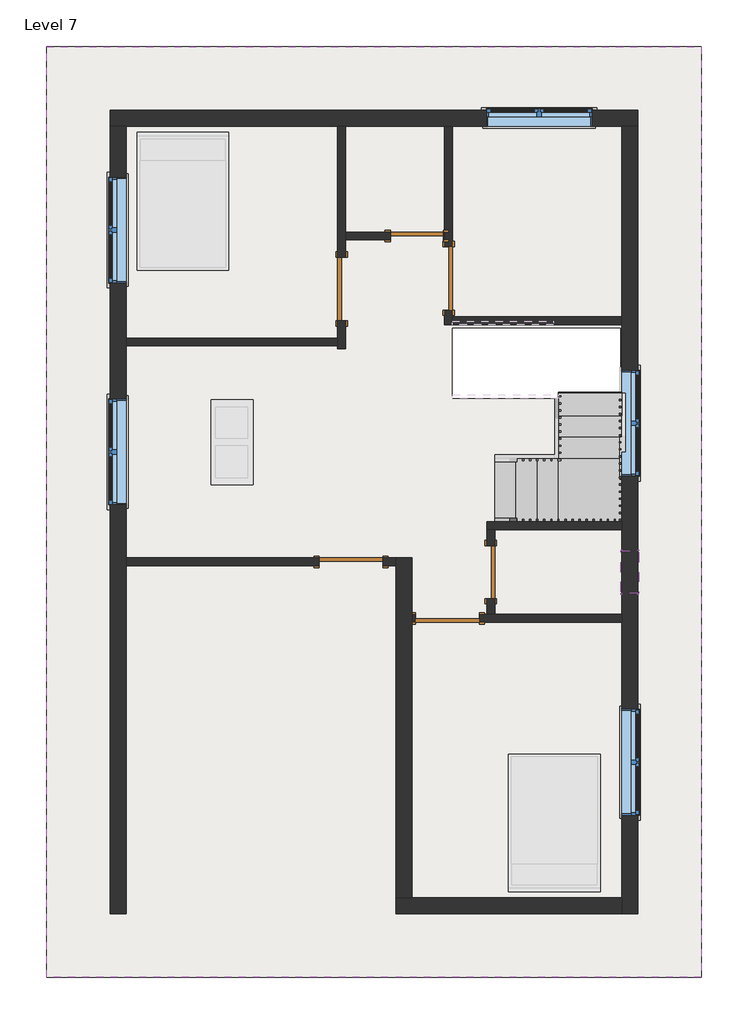
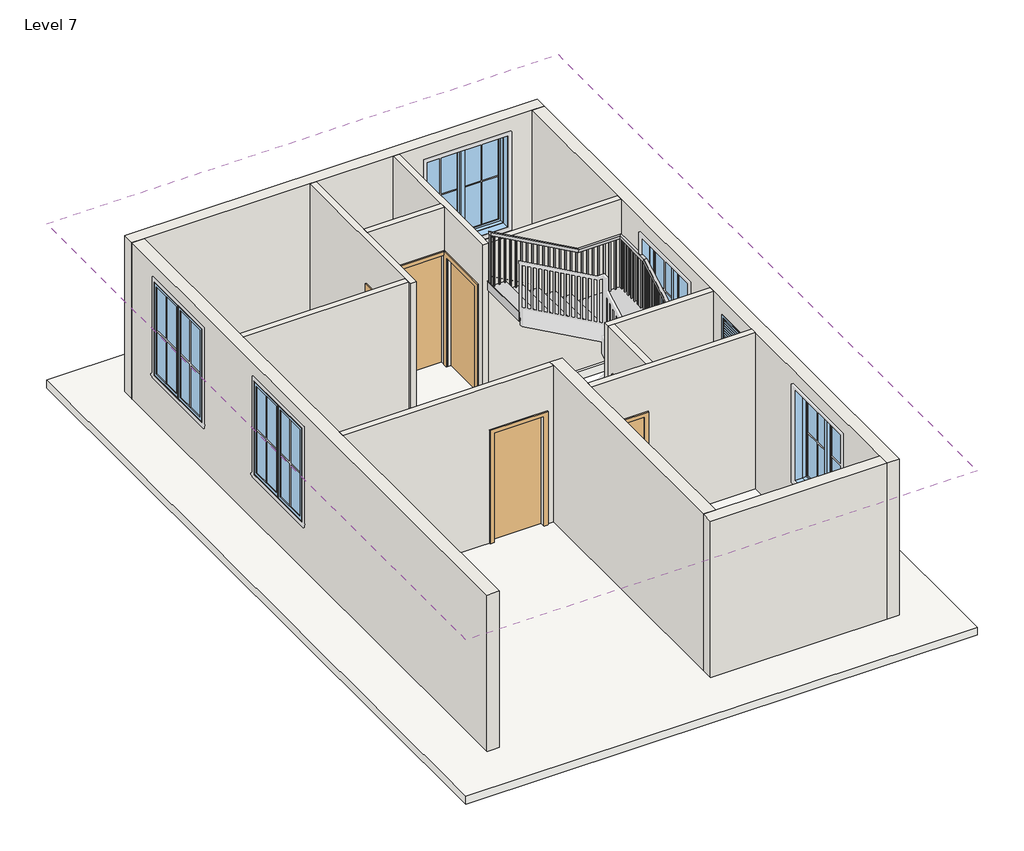
# One storey, part 1 of 2: 14 walls, 6 doors, 6 windows, 2 roofs, 1 railing, 1 slab, 1 stair flight.
"""IFC4 building model written with IfcOpenShell, lengths in millimetres."""

from ifc_helpers import new_model, si_unit, frame, origin, place, context, project, spatial, polyline, outline, extrude, faceted_brep, transform, mapped, element, save
from components import door_214872d5, door_78caadf7, single_flush_door_3_e5f9f3c4, single_flush_door_3_305aa2a5, stair_flight_68b2e5de, window_casement_double_win_5_f93960c7, window_f2d8fef0

model = new_model("IFC4")

# Units and contexts
model_context = context("Model", 3, world=origin())
ifc_project = project(units=[si_unit("LENGTHUNIT", "METRE", prefix="MILLI")], contexts=[model_context])

# Site, building, storey
site = spatial("IfcSite", under=ifc_project)
building = spatial("IfcBuilding", under=site)
storey = spatial("IfcBuildingStorey", under=building, Name="Level 7", Elevation=16002.0)

# Doors
placement = place(None, origin())
door_shape = door_214872d5(model_context)
element("IfcDoor", 1, ObjectType="Single-Flush : DOOR 2'6\"", at=placement, inside=storey, context=model_context, shape_type="MappedRepresentation", body=[
    mapped(door_shape, transform((-185.4325206, 3926.3629493, 16002.0), x_axis=(1.0, 0.0, 0.0), y_axis=(0.0, 1.0, 0.0), z_axis=(0.0, 0.0, 1.0))),
])
door_2_shape = door_78caadf7(model_context)
element("IfcDoor", 2, ObjectType="Single-Flush : DOOR 2'6\"", at=placement, inside=storey, context=model_context, shape_type="MappedRepresentation", body=[
    mapped(door_2_shape, transform((881.3674794, -905.9870507, 16002.0), x_axis=(0.0, 1.0, 0.0), y_axis=(-1.0, 0.0, 0.0), z_axis=(0.0, 0.0, 1.0))),
])
single_flush_door_3_shape = single_flush_door_3_e5f9f3c4(model_context)
element("IfcDoor", 3, ObjectType="Single-Flush : DOOR 3'", at=placement, inside=storey, context=model_context, shape_type="MappedRepresentation", body=[
    mapped(single_flush_door_3_shape, transform((271.7674794, 3316.7629493, 16002.0), x_axis=(0.0, -1.0, 0.0), y_axis=(1.0, 0.0, 0.0), z_axis=(0.0, 0.0, 1.0))),
])
element("IfcDoor", 4, ObjectType="Single-Flush : DOOR 3'", at=placement, inside=storey, context=model_context, shape_type="MappedRepresentation", body=[
    mapped(single_flush_door_3_shape, transform((255.8924794, -1572.7370507, 16002.0), x_axis=(-1.0, 0.0, 0.0), y_axis=(0.0, -1.0, 0.0), z_axis=(0.0, 0.0, 1.0))),
])
single_flush_door_3_2_shape = single_flush_door_3_305aa2a5(model_context)
element("IfcDoor", 5, ObjectType="Single-Flush : DOOR 3'", at=placement, inside=storey, context=model_context, shape_type="MappedRepresentation", body=[
    mapped(single_flush_door_3_2_shape, transform((-1264.9325206, 3164.3629493, 16002.0), x_axis=(0.0, -1.0, 0.0), y_axis=(1.0, 0.0, 0.0), z_axis=(0.0, 0.0, 1.0))),
])
element("IfcDoor", 6, ObjectType="Single-Flush : DOOR 3'6\"", at=placement, inside=storey, context=model_context, shape_type="MappedRepresentation", body=[
    mapped(single_flush_door_3_shape, transform((-1131.5825206, -759.9370507, 16002.0), x_axis=(1.0, 0.0, 0.0), y_axis=(0.0, 1.0, 0.0), z_axis=(0.0, 0.0, 1.0))),
])

# Railing
element("IfcRailing", 7, ObjectType="Handrail - Rectangular", at=placement, inside=storey, context=model_context, shape_type="SolidModel", body=[
    faceted_brep([(938.5174794, -131.2870507, 17085.7333333), (938.5174794, -131.2870507, 17027.620221), (938.5174794, -182.0870507, 17027.620221), (938.5174794, -182.0870507, 17085.7333333), (2005.3174794, -131.2870507, 17678.4), (2018.4810817, -131.2870507, 17627.6), (2018.4810817, -182.0870507, 17627.6), (2005.3174794, -182.0870507, 17678.4), (2716.5174794, -131.2870507, 17678.4), (2716.5174794, -131.2870507, 17627.6), (2767.3174794, -182.0870507, 17627.6), (2767.3174794, -182.0870507, 17678.4), (2716.5174794, 579.9129493, 17678.4), (2716.5174794, 593.0765516, 17627.6), (2767.3174794, 593.0765516, 17627.6), (2767.3174794, 579.9129493, 17678.4), (2716.5174794, 1843.5629493, 18380.4277778), (2716.5174794, 1856.7265516, 18329.6277778), (2767.3174794, 1856.7265516, 18329.6277778), (2767.3174794, 1843.5629493, 18380.4277778), (2716.5174794, 2599.2129493, 18380.4277778), (2716.5174794, 2599.2129493, 18329.6277778), (2767.3174794, 2650.0129493, 18329.6277778), (2767.3174794, 2650.0129493, 18380.4277778), (1960.8674794, 2599.2129493, 18380.4277778), (1947.7038772, 2599.2129493, 18329.6277778), (1947.7038772, 2650.0129493, 18329.6277778), (1960.8674794, 2650.0129493, 18380.4277778), (328.9174794, 2599.2129493, 19287.0666667), (328.9174794, 2650.0129493, 19287.0666667), (328.9174794, 2650.0129493, 19228.9535543), (328.9174794, 2599.2129493, 19228.9535543)], [[[0, 1, 2, 3]], [[1, 0, 4, 5]], [[2, 1, 5, 6]], [[3, 2, 6, 7]], [[0, 3, 7, 4]], [[5, 4, 8, 9]], [[6, 5, 9, 10]], [[7, 6, 10, 11]], [[4, 7, 11, 8]], [[9, 8, 12, 13]], [[10, 9, 13, 14]], [[11, 10, 14, 15]], [[8, 11, 15, 12]], [[13, 12, 16, 17]], [[14, 13, 17, 18]], [[15, 14, 18, 19]], [[12, 15, 19, 16]], [[17, 16, 20, 21]], [[18, 17, 21, 22]], [[19, 18, 22, 23]], [[16, 19, 23, 20]], [[21, 20, 24, 25]], [[22, 21, 25, 26]], [[23, 22, 26, 27]], [[20, 23, 27, 24]], [[28, 29, 30, 31]], [[25, 24, 28, 31]], [[26, 25, 31, 30]], [[27, 26, 30, 29]], [[24, 27, 29, 28]]]),
    extrude(outline(polyline([(19181.3285543, 414.6424794), (19191.9118876, 395.5924794), (18203.3333333, 395.5924794), (18203.3333333, 414.6424794), (19181.3285543, 414.6424794)])), frame((0.0, 2615.0879493, 0.0), z_axis=(0.0, 1.0, 0.0), x_axis=(0.0, 0.0, 1.0)), (0.0, 0.0, 1.0), 19.05),
    extrude(outline(polyline([(19124.8841099, 516.2424794), (19135.4674432, 497.1924794), (18203.3333333, 497.1924794), (18203.3333333, 516.2424794), (19124.8841099, 516.2424794)])), frame((0.0, 2615.0879493, 0.0), z_axis=(0.0, 1.0, 0.0), x_axis=(0.0, 0.0, 1.0)), (0.0, 0.0, 1.0), 19.05),
    extrude(outline(polyline([(19068.4396654, 617.8424794), (19079.0229988, 598.7924794), (18203.3333333, 598.7924794), (18203.3333333, 617.8424794), (19068.4396654, 617.8424794)])), frame((0.0, 2615.0879493, 0.0), z_axis=(0.0, 1.0, 0.0), x_axis=(0.0, 0.0, 1.0)), (0.0, 0.0, 1.0), 19.05),
    extrude(outline(polyline([(19011.995221, 719.4424794), (19022.5785543, 700.3924794), (18034.0, 700.3924794), (18034.0, 719.4424794), (19011.995221, 719.4424794)])), frame((0.0, 2615.0879493, 0.0), z_axis=(0.0, 1.0, 0.0), x_axis=(0.0, 0.0, 1.0)), (0.0, 0.0, 1.0), 19.05),
    extrude(outline(polyline([(18955.5507765, 821.0424794), (18966.1341099, 801.9924794), (18034.0, 801.9924794), (18034.0, 821.0424794), (18955.5507765, 821.0424794)])), frame((0.0, 2615.0879493, 0.0), z_axis=(0.0, 1.0, 0.0), x_axis=(0.0, 0.0, 1.0)), (0.0, 0.0, 1.0), 19.05),
    extrude(outline(polyline([(18899.1063321, 922.6424794), (18909.6896654, 903.5924794), (18034.0, 903.5924794), (18034.0, 922.6424794), (18899.1063321, 922.6424794)])), frame((0.0, 2615.0879493, 0.0), z_axis=(0.0, 1.0, 0.0), x_axis=(0.0, 0.0, 1.0)), (0.0, 0.0, 1.0), 19.05),
    extrude(outline(polyline([(18842.6618876, 1024.2424794), (18853.245221, 1005.1924794), (17864.6666667, 1005.1924794), (17864.6666667, 1024.2424794), (18842.6618876, 1024.2424794)])), frame((0.0, 2615.0879493, 0.0), z_axis=(0.0, 1.0, 0.0), x_axis=(0.0, 0.0, 1.0)), (0.0, 0.0, 1.0), 19.05),
    extrude(outline(polyline([(18786.2174432, 1125.8424794), (18796.8007765, 1106.7924794), (17864.6666667, 1106.7924794), (17864.6666667, 1125.8424794), (18786.2174432, 1125.8424794)])), frame((0.0, 2615.0879493, 0.0), z_axis=(0.0, 1.0, 0.0), x_axis=(0.0, 0.0, 1.0)), (0.0, 0.0, 1.0), 19.05),
    extrude(outline(polyline([(18729.7729988, 1227.4424794), (18740.3563321, 1208.3924794), (17864.6666667, 1208.3924794), (17864.6666667, 1227.4424794), (18729.7729988, 1227.4424794)])), frame((0.0, 2615.0879493, 0.0), z_axis=(0.0, 1.0, 0.0), x_axis=(0.0, 0.0, 1.0)), (0.0, 0.0, 1.0), 19.05),
    extrude(outline(polyline([(18673.3285543, 1329.0424794), (18683.9118876, 1309.9924794), (17695.3333333, 1309.9924794), (17695.3333333, 1329.0424794), (18673.3285543, 1329.0424794)])), frame((0.0, 2615.0879493, 0.0), z_axis=(0.0, 1.0, 0.0), x_axis=(0.0, 0.0, 1.0)), (0.0, 0.0, 1.0), 19.05),
    extrude(outline(polyline([(18616.8841099, 1430.6424794), (18627.4674432, 1411.5924794), (17695.3333333, 1411.5924794), (17695.3333333, 1430.6424794), (18616.8841099, 1430.6424794)])), frame((0.0, 2615.0879493, 0.0), z_axis=(0.0, 1.0, 0.0), x_axis=(0.0, 0.0, 1.0)), (0.0, 0.0, 1.0), 19.05),
    extrude(outline(polyline([(18560.4396654, 1532.2424794), (18571.0229988, 1513.1924794), (17695.3333333, 1513.1924794), (17695.3333333, 1532.2424794), (18560.4396654, 1532.2424794)])), frame((0.0, 2615.0879493, 0.0), z_axis=(0.0, 1.0, 0.0), x_axis=(0.0, 0.0, 1.0)), (0.0, 0.0, 1.0), 19.05),
    extrude(outline(polyline([(18503.995221, 1633.8424794), (18514.5785543, 1614.7924794), (17526.0, 1614.7924794), (17526.0, 1633.8424794), (18503.995221, 1633.8424794)])), frame((0.0, 2615.0879493, 0.0), z_axis=(0.0, 1.0, 0.0), x_axis=(0.0, 0.0, 1.0)), (0.0, 0.0, 1.0), 19.05),
    extrude(outline(polyline([(18447.5507765, 1735.4424794), (18458.1341099, 1716.3924794), (17526.0, 1716.3924794), (17526.0, 1735.4424794), (18447.5507765, 1735.4424794)])), frame((0.0, 2615.0879493, 0.0), z_axis=(0.0, 1.0, 0.0), x_axis=(0.0, 0.0, 1.0)), (0.0, 0.0, 1.0), 19.05),
    extrude(outline(polyline([(18391.1063321, 1837.0424794), (18401.6896654, 1817.9924794), (17526.0, 1817.9924794), (17526.0, 1837.0424794), (18391.1063321, 1837.0424794)])), frame((0.0, 2615.0879493, 0.0), z_axis=(0.0, 1.0, 0.0), x_axis=(0.0, 0.0, 1.0)), (0.0, 0.0, 1.0), 19.05),
    extrude(outline(polyline([(18334.6618876, 1938.6424794), (18345.245221, 1919.5924794), (17356.6666667, 1919.5924794), (17356.6666667, 1938.6424794), (18334.6618876, 1938.6424794)])), frame((0.0, 2615.0879493, 0.0), z_axis=(0.0, 1.0, 0.0), x_axis=(0.0, 0.0, 1.0)), (0.0, 0.0, 1.0), 19.05),
    extrude(outline(polyline([(2040.2424794, 2634.1379493), (2040.2424794, 2615.0879493), (2021.1924794, 2615.0879493), (2021.1924794, 2634.1379493), (2040.2424794, 2634.1379493)])), frame((0.0, 0.0, 17356.6666667), z_axis=(0.0, 0.0, 1.0), x_axis=(1.0, 0.0, 0.0)), (0.0, 0.0, 1.0), 972.9611111),
    extrude(outline(polyline([(2141.8424794, 2634.1379493), (2141.8424794, 2615.0879493), (2122.7924794, 2615.0879493), (2122.7924794, 2634.1379493), (2141.8424794, 2634.1379493)])), frame((0.0, 0.0, 17356.6666667), z_axis=(0.0, 0.0, 1.0), x_axis=(1.0, 0.0, 0.0)), (0.0, 0.0, 1.0), 972.9611111),
    extrude(outline(polyline([(2243.4424794, 2634.1379493), (2243.4424794, 2615.0879493), (2224.3924794, 2615.0879493), (2224.3924794, 2634.1379493), (2243.4424794, 2634.1379493)])), frame((0.0, 0.0, 17356.6666667), z_axis=(0.0, 0.0, 1.0), x_axis=(1.0, 0.0, 0.0)), (0.0, 0.0, 1.0), 972.9611111),
    extrude(outline(polyline([(2345.0424794, 2634.1379493), (2345.0424794, 2615.0879493), (2325.9924794, 2615.0879493), (2325.9924794, 2634.1379493), (2345.0424794, 2634.1379493)])), frame((0.0, 0.0, 17356.6666667), z_axis=(0.0, 0.0, 1.0), x_axis=(1.0, 0.0, 0.0)), (0.0, 0.0, 1.0), 972.9611111),
    extrude(outline(polyline([(2446.6424794, 2634.1379493), (2446.6424794, 2615.0879493), (2427.5924794, 2615.0879493), (2427.5924794, 2634.1379493), (2446.6424794, 2634.1379493)])), frame((0.0, 0.0, 17356.6666667), z_axis=(0.0, 0.0, 1.0), x_axis=(1.0, 0.0, 0.0)), (0.0, 0.0, 1.0), 972.9611111),
    extrude(outline(polyline([(2548.2424794, 2634.1379493), (2548.2424794, 2615.0879493), (2529.1924794, 2615.0879493), (2529.1924794, 2634.1379493), (2548.2424794, 2634.1379493)])), frame((0.0, 0.0, 17356.6666667), z_axis=(0.0, 0.0, 1.0), x_axis=(1.0, 0.0, 0.0)), (0.0, 0.0, 1.0), 972.9611111),
    extrude(outline(polyline([(2649.8424794, 2634.1379493), (2649.8424794, 2615.0879493), (2630.7924794, 2615.0879493), (2630.7924794, 2634.1379493), (2649.8424794, 2634.1379493)])), frame((0.0, 0.0, 17356.6666667), z_axis=(0.0, 0.0, 1.0), x_axis=(1.0, 0.0, 0.0)), (0.0, 0.0, 1.0), 972.9611111),
    extrude(outline(polyline([(2751.4424794, 2576.9879493), (2732.3924794, 2576.9879493), (2732.3924794, 2596.0379493), (2751.4424794, 2596.0379493), (2751.4424794, 2576.9879493)])), frame((0.0, 0.0, 17356.6666667), z_axis=(0.0, 0.0, 1.0), x_axis=(1.0, 0.0, 0.0)), (0.0, 0.0, 1.0), 972.9611111),
    extrude(outline(polyline([(2751.4424794, 2475.3879493), (2732.3924794, 2475.3879493), (2732.3924794, 2494.4379493), (2751.4424794, 2494.4379493), (2751.4424794, 2475.3879493)])), frame((0.0, 0.0, 17356.6666667), z_axis=(0.0, 0.0, 1.0), x_axis=(1.0, 0.0, 0.0)), (0.0, 0.0, 1.0), 972.9611111),
    extrude(outline(polyline([(2751.4424794, 2373.7879493), (2732.3924794, 2373.7879493), (2732.3924794, 2392.8379493), (2751.4424794, 2392.8379493), (2751.4424794, 2373.7879493)])), frame((0.0, 0.0, 17356.6666667), z_axis=(0.0, 0.0, 1.0), x_axis=(1.0, 0.0, 0.0)), (0.0, 0.0, 1.0), 972.9611111),
    extrude(outline(polyline([(2751.4424794, 2272.1879493), (2732.3924794, 2272.1879493), (2732.3924794, 2291.2379493), (2751.4424794, 2291.2379493), (2751.4424794, 2272.1879493)])), frame((0.0, 0.0, 17356.6666667), z_axis=(0.0, 0.0, 1.0), x_axis=(1.0, 0.0, 0.0)), (0.0, 0.0, 1.0), 972.9611111),
    extrude(outline(polyline([(2751.4424794, 2170.5879493), (2732.3924794, 2170.5879493), (2732.3924794, 2189.6379493), (2751.4424794, 2189.6379493), (2751.4424794, 2170.5879493)])), frame((0.0, 0.0, 17356.6666667), z_axis=(0.0, 0.0, 1.0), x_axis=(1.0, 0.0, 0.0)), (0.0, 0.0, 1.0), 972.9611111),
    extrude(outline(polyline([(2751.4424794, 2068.9879493), (2732.3924794, 2068.9879493), (2732.3924794, 2088.0379493), (2751.4424794, 2088.0379493), (2751.4424794, 2068.9879493)])), frame((0.0, 0.0, 17356.6666667), z_axis=(0.0, 0.0, 1.0), x_axis=(1.0, 0.0, 0.0)), (0.0, 0.0, 1.0), 972.9611111),
    extrude(outline(polyline([(2751.4424794, 1967.3879493), (2732.3924794, 1967.3879493), (2732.3924794, 1986.4379493), (2751.4424794, 1986.4379493), (2751.4424794, 1967.3879493)])), frame((0.0, 0.0, 17356.6666667), z_axis=(0.0, 0.0, 1.0), x_axis=(1.0, 0.0, 0.0)), (0.0, 0.0, 1.0), 972.9611111),
    extrude(outline(polyline([(2751.4424794, 1865.7879493), (2732.3924794, 1865.7879493), (2732.3924794, 1884.8379493), (2751.4424794, 1884.8379493), (2751.4424794, 1865.7879493)])), frame((0.0, 0.0, 17356.6666667), z_axis=(0.0, 0.0, 1.0), x_axis=(1.0, 0.0, 0.0)), (0.0, 0.0, 1.0), 972.9611111),
    extrude(outline(polyline([(1764.1879493, 18278.2174432), (1783.2379493, 18288.8007765), (1783.2379493, 17356.6666667), (1764.1879493, 17356.6666667), (1764.1879493, 18278.2174432)])), frame((2732.3924794, 0.0, 0.0), z_axis=(1.0, 0.0, 0.0), x_axis=(0.0, 1.0, 0.0)), (0.0, 0.0, 1.0), 19.05),
    extrude(outline(polyline([(1662.5879493, 18221.7729988), (1681.6379493, 18232.3563321), (1681.6379493, 17356.6666667), (1662.5879493, 17356.6666667), (1662.5879493, 18221.7729988)])), frame((2732.3924794, 0.0, 0.0), z_axis=(1.0, 0.0, 0.0), x_axis=(0.0, 1.0, 0.0)), (0.0, 0.0, 1.0), 19.05),
    extrude(outline(polyline([(1560.9879493, 18165.3285543), (1580.0379493, 18175.9118876), (1580.0379493, 17187.3333333), (1560.9879493, 17187.3333333), (1560.9879493, 18165.3285543)])), frame((2732.3924794, 0.0, 0.0), z_axis=(1.0, 0.0, 0.0), x_axis=(0.0, 1.0, 0.0)), (0.0, 0.0, 1.0), 19.05),
    extrude(outline(polyline([(1459.3879493, 18108.8841099), (1478.4379493, 18119.4674432), (1478.4379493, 17187.3333333), (1459.3879493, 17187.3333333), (1459.3879493, 18108.8841099)])), frame((2732.3924794, 0.0, 0.0), z_axis=(1.0, 0.0, 0.0), x_axis=(0.0, 1.0, 0.0)), (0.0, 0.0, 1.0), 19.05),
    extrude(outline(polyline([(1357.7879493, 18052.4396654), (1376.8379493, 18063.0229988), (1376.8379493, 17187.3333333), (1357.7879493, 17187.3333333), (1357.7879493, 18052.4396654)])), frame((2732.3924794, 0.0, 0.0), z_axis=(1.0, 0.0, 0.0), x_axis=(0.0, 1.0, 0.0)), (0.0, 0.0, 1.0), 19.05),
    extrude(outline(polyline([(1256.1879493, 17995.995221), (1275.2379493, 18006.5785543), (1275.2379493, 17018.0), (1256.1879493, 17018.0), (1256.1879493, 17995.995221)])), frame((2732.3924794, 0.0, 0.0), z_axis=(1.0, 0.0, 0.0), x_axis=(0.0, 1.0, 0.0)), (0.0, 0.0, 1.0), 19.05),
    extrude(outline(polyline([(1154.5879493, 17939.5507765), (1173.6379493, 17950.1341099), (1173.6379493, 17018.0), (1154.5879493, 17018.0), (1154.5879493, 17939.5507765)])), frame((2732.3924794, 0.0, 0.0), z_axis=(1.0, 0.0, 0.0), x_axis=(0.0, 1.0, 0.0)), (0.0, 0.0, 1.0), 19.05),
    extrude(outline(polyline([(1052.9879493, 17883.1063321), (1072.0379493, 17893.6896654), (1072.0379493, 17018.0), (1052.9879493, 17018.0), (1052.9879493, 17883.1063321)])), frame((2732.3924794, 0.0, 0.0), z_axis=(1.0, 0.0, 0.0), x_axis=(0.0, 1.0, 0.0)), (0.0, 0.0, 1.0), 19.05),
    extrude(outline(polyline([(951.3879493, 17826.6618876), (970.4379493, 17837.245221), (970.4379493, 16848.6666667), (951.3879493, 16848.6666667), (951.3879493, 17826.6618876)])), frame((2732.3924794, 0.0, 0.0), z_axis=(1.0, 0.0, 0.0), x_axis=(0.0, 1.0, 0.0)), (0.0, 0.0, 1.0), 19.05),
    extrude(outline(polyline([(849.7879493, 17770.2174432), (868.8379493, 17780.8007765), (868.8379493, 16848.6666667), (849.7879493, 16848.6666667), (849.7879493, 17770.2174432)])), frame((2732.3924794, 0.0, 0.0), z_axis=(1.0, 0.0, 0.0), x_axis=(0.0, 1.0, 0.0)), (0.0, 0.0, 1.0), 19.05),
    extrude(outline(polyline([(748.1879493, 17713.7729988), (767.2379493, 17724.3563321), (767.2379493, 16848.6666667), (748.1879493, 16848.6666667), (748.1879493, 17713.7729988)])), frame((2732.3924794, 0.0, 0.0), z_axis=(1.0, 0.0, 0.0), x_axis=(0.0, 1.0, 0.0)), (0.0, 0.0, 1.0), 19.05),
    extrude(outline(polyline([(646.5879493, 17657.3285543), (665.6379493, 17667.9118876), (665.6379493, 16679.3333333), (646.5879493, 16679.3333333), (646.5879493, 17657.3285543)])), frame((2732.3924794, 0.0, 0.0), z_axis=(1.0, 0.0, 0.0), x_axis=(0.0, 1.0, 0.0)), (0.0, 0.0, 1.0), 19.05),
    extrude(outline(polyline([(2751.4424794, 544.9879493), (2732.3924794, 544.9879493), (2732.3924794, 564.0379493), (2751.4424794, 564.0379493), (2751.4424794, 544.9879493)])), frame((0.0, 0.0, 16679.3333333), z_axis=(0.0, 0.0, 1.0), x_axis=(1.0, 0.0, 0.0)), (0.0, 0.0, 1.0), 948.2666667),
    extrude(outline(polyline([(2751.4424794, 443.3879493), (2732.3924794, 443.3879493), (2732.3924794, 462.4379493), (2751.4424794, 462.4379493), (2751.4424794, 443.3879493)])), frame((0.0, 0.0, 16679.3333333), z_axis=(0.0, 0.0, 1.0), x_axis=(1.0, 0.0, 0.0)), (0.0, 0.0, 1.0), 948.2666667),
    extrude(outline(polyline([(2751.4424794, 341.7879493), (2732.3924794, 341.7879493), (2732.3924794, 360.8379493), (2751.4424794, 360.8379493), (2751.4424794, 341.7879493)])), frame((0.0, 0.0, 16679.3333333), z_axis=(0.0, 0.0, 1.0), x_axis=(1.0, 0.0, 0.0)), (0.0, 0.0, 1.0), 948.2666667),
    extrude(outline(polyline([(2751.4424794, 240.1879493), (2732.3924794, 240.1879493), (2732.3924794, 259.2379493), (2751.4424794, 259.2379493), (2751.4424794, 240.1879493)])), frame((0.0, 0.0, 16679.3333333), z_axis=(0.0, 0.0, 1.0), x_axis=(1.0, 0.0, 0.0)), (0.0, 0.0, 1.0), 948.2666667),
    extrude(outline(polyline([(2751.4424794, 138.5879493), (2732.3924794, 138.5879493), (2732.3924794, 157.6379493), (2751.4424794, 157.6379493), (2751.4424794, 138.5879493)])), frame((0.0, 0.0, 16679.3333333), z_axis=(0.0, 0.0, 1.0), x_axis=(1.0, 0.0, 0.0)), (0.0, 0.0, 1.0), 948.2666667),
    extrude(outline(polyline([(2751.4424794, 36.9879493), (2732.3924794, 36.9879493), (2732.3924794, 56.0379493), (2751.4424794, 56.0379493), (2751.4424794, 36.9879493)])), frame((0.0, 0.0, 16679.3333333), z_axis=(0.0, 0.0, 1.0), x_axis=(1.0, 0.0, 0.0)), (0.0, 0.0, 1.0), 948.2666667),
    extrude(outline(polyline([(2751.4424794, -64.6120507), (2732.3924794, -64.6120507), (2732.3924794, -45.5620507), (2751.4424794, -45.5620507), (2751.4424794, -64.6120507)])), frame((0.0, 0.0, 16679.3333333), z_axis=(0.0, 0.0, 1.0), x_axis=(1.0, 0.0, 0.0)), (0.0, 0.0, 1.0), 948.2666667),
    extrude(outline(polyline([(2656.1924794, -166.2120507), (2656.1924794, -147.1620507), (2675.2424794, -147.1620507), (2675.2424794, -166.2120507), (2656.1924794, -166.2120507)])), frame((0.0, 0.0, 16679.3333333), z_axis=(0.0, 0.0, 1.0), x_axis=(1.0, 0.0, 0.0)), (0.0, 0.0, 1.0), 948.2666667),
    extrude(outline(polyline([(2554.5924794, -166.2120507), (2554.5924794, -147.1620507), (2573.6424794, -147.1620507), (2573.6424794, -166.2120507), (2554.5924794, -166.2120507)])), frame((0.0, 0.0, 16679.3333333), z_axis=(0.0, 0.0, 1.0), x_axis=(1.0, 0.0, 0.0)), (0.0, 0.0, 1.0), 948.2666667),
    extrude(outline(polyline([(2452.9924794, -166.2120507), (2452.9924794, -147.1620507), (2472.0424794, -147.1620507), (2472.0424794, -166.2120507), (2452.9924794, -166.2120507)])), frame((0.0, 0.0, 16679.3333333), z_axis=(0.0, 0.0, 1.0), x_axis=(1.0, 0.0, 0.0)), (0.0, 0.0, 1.0), 948.2666667),
    extrude(outline(polyline([(2351.3924794, -166.2120507), (2351.3924794, -147.1620507), (2370.4424794, -147.1620507), (2370.4424794, -166.2120507), (2351.3924794, -166.2120507)])), frame((0.0, 0.0, 16679.3333333), z_axis=(0.0, 0.0, 1.0), x_axis=(1.0, 0.0, 0.0)), (0.0, 0.0, 1.0), 948.2666667),
    extrude(outline(polyline([(2249.7924794, -166.2120507), (2249.7924794, -147.1620507), (2268.8424794, -147.1620507), (2268.8424794, -166.2120507), (2249.7924794, -166.2120507)])), frame((0.0, 0.0, 16679.3333333), z_axis=(0.0, 0.0, 1.0), x_axis=(1.0, 0.0, 0.0)), (0.0, 0.0, 1.0), 948.2666667),
    extrude(outline(polyline([(2148.1924794, -166.2120507), (2148.1924794, -147.1620507), (2167.2424794, -147.1620507), (2167.2424794, -166.2120507), (2148.1924794, -166.2120507)])), frame((0.0, 0.0, 16679.3333333), z_axis=(0.0, 0.0, 1.0), x_axis=(1.0, 0.0, 0.0)), (0.0, 0.0, 1.0), 948.2666667),
    extrude(outline(polyline([(2046.5924794, -166.2120507), (2046.5924794, -147.1620507), (2065.6424794, -147.1620507), (2065.6424794, -166.2120507), (2046.5924794, -166.2120507)])), frame((0.0, 0.0, 16679.3333333), z_axis=(0.0, 0.0, 1.0), x_axis=(1.0, 0.0, 0.0)), (0.0, 0.0, 1.0), 948.2666667),
    extrude(outline(polyline([(17597.3563321, 1964.0424794), (17586.7729988, 1944.9924794), (16679.3333333, 1944.9924794), (16679.3333333, 1964.0424794), (17597.3563321, 1964.0424794)])), frame((0.0, -166.2120507, 0.0), z_axis=(0.0, 1.0, 0.0), x_axis=(0.0, 0.0, 1.0)), (0.0, 0.0, 1.0), 19.05),
    extrude(outline(polyline([(17540.9118876, 1862.4424794), (17530.3285543, 1843.3924794), (16679.3333333, 1843.3924794), (16679.3333333, 1862.4424794), (17540.9118876, 1862.4424794)])), frame((0.0, -166.2120507, 0.0), z_axis=(0.0, 1.0, 0.0), x_axis=(0.0, 0.0, 1.0)), (0.0, 0.0, 1.0), 19.05),
    extrude(outline(polyline([(17484.4674432, 1760.8424794), (17473.8841099, 1741.7924794), (16510.0, 1741.7924794), (16510.0, 1760.8424794), (17484.4674432, 1760.8424794)])), frame((0.0, -166.2120507, 0.0), z_axis=(0.0, 1.0, 0.0), x_axis=(0.0, 0.0, 1.0)), (0.0, 0.0, 1.0), 19.05),
    extrude(outline(polyline([(17428.0229988, 1659.2424794), (17417.4396654, 1640.1924794), (16510.0, 1640.1924794), (16510.0, 1659.2424794), (17428.0229988, 1659.2424794)])), frame((0.0, -166.2120507, 0.0), z_axis=(0.0, 1.0, 0.0), x_axis=(0.0, 0.0, 1.0)), (0.0, 0.0, 1.0), 19.05),
    extrude(outline(polyline([(17371.5785543, 1557.6424794), (17360.995221, 1538.5924794), (16510.0, 1538.5924794), (16510.0, 1557.6424794), (17371.5785543, 1557.6424794)])), frame((0.0, -166.2120507, 0.0), z_axis=(0.0, 1.0, 0.0), x_axis=(0.0, 0.0, 1.0)), (0.0, 0.0, 1.0), 19.05),
    extrude(outline(polyline([(17315.1341099, 1456.0424794), (17304.5507765, 1436.9924794), (16340.6666667, 1436.9924794), (16340.6666667, 1456.0424794), (17315.1341099, 1456.0424794)])), frame((0.0, -166.2120507, 0.0), z_axis=(0.0, 1.0, 0.0), x_axis=(0.0, 0.0, 1.0)), (0.0, 0.0, 1.0), 19.05),
    extrude(outline(polyline([(17258.6896654, 1354.4424794), (17248.1063321, 1335.3924794), (16340.6666667, 1335.3924794), (16340.6666667, 1354.4424794), (17258.6896654, 1354.4424794)])), frame((0.0, -166.2120507, 0.0), z_axis=(0.0, 1.0, 0.0), x_axis=(0.0, 0.0, 1.0)), (0.0, 0.0, 1.0), 19.05),
    extrude(outline(polyline([(17202.245221, 1252.8424794), (17191.6618876, 1233.7924794), (16340.6666667, 1233.7924794), (16340.6666667, 1252.8424794), (17202.245221, 1252.8424794)])), frame((0.0, -166.2120507, 0.0), z_axis=(0.0, 1.0, 0.0), x_axis=(0.0, 0.0, 1.0)), (0.0, 0.0, 1.0), 19.05),
    extrude(outline(polyline([(17145.8007765, 1151.2424794), (17135.2174432, 1132.1924794), (16171.3333333, 1132.1924794), (16171.3333333, 1151.2424794), (17145.8007765, 1151.2424794)])), frame((0.0, -166.2120507, 0.0), z_axis=(0.0, 1.0, 0.0), x_axis=(0.0, 0.0, 1.0)), (0.0, 0.0, 1.0), 19.05),
    extrude(outline(polyline([(17089.3563321, 1049.6424794), (17078.7729988, 1030.5924794), (16171.3333333, 1030.5924794), (16171.3333333, 1049.6424794), (17089.3563321, 1049.6424794)])), frame((0.0, -166.2120507, 0.0), z_axis=(0.0, 1.0, 0.0), x_axis=(0.0, 0.0, 1.0)), (0.0, 0.0, 1.0), 19.05),
    extrude(outline(polyline([(2751.4424794, 2615.0879493), (2732.3924794, 2615.0879493), (2732.3924794, 2634.1379493), (2751.4424794, 2634.1379493), (2751.4424794, 2615.0879493)])), frame((0.0, 0.0, 17356.6666667), z_axis=(0.0, 0.0, 1.0), x_axis=(1.0, 0.0, 0.0)), (0.0, 0.0, 1.0), 972.9611111),
    extrude(outline(polyline([(2732.3924794, -166.2120507), (2732.3924794, -147.1620507), (2751.4424794, -147.1620507), (2751.4424794, -166.2120507), (2732.3924794, -166.2120507)])), frame((0.0, 0.0, 16679.3333333), z_axis=(0.0, 0.0, 1.0), x_axis=(1.0, 0.0, 0.0)), (0.0, 0.0, 1.0), 948.2666667),
    extrude(outline(polyline([(19218.370221, 347.9674794), (19228.9535543, 328.9174794), (18203.3333333, 328.9174794), (18203.3333333, 347.9674794), (19218.370221, 347.9674794)])), frame((0.0, 2615.0879493, 0.0), z_axis=(0.0, 1.0, 0.0), x_axis=(0.0, 0.0, 1.0)), (0.0, 0.0, 1.0), 19.05),
    extrude(outline(polyline([(17038.2035543, 957.5674794), (17027.620221, 938.5174794), (16171.3333333, 938.5174794), (16171.3333333, 957.5674794), (17038.2035543, 957.5674794)])), frame((0.0, -166.2120507, 0.0), z_axis=(0.0, 1.0, 0.0), x_axis=(0.0, 0.0, 1.0)), (0.0, 0.0, 1.0), 19.05),
])

# Roofs
element("IfcRoof", 8, ObjectType="ROOF 6\"", at=placement, inside=storey, context=model_context, shape_type="SweptSolid", body=[
    extrude(outline(polyline([(-5513.0825206, 6650.5129493), (3910.3174794, 6650.5129493), (3910.3174794, -6735.2870507), (-5513.0825206, -6735.2870507), (-5513.0825206, 6650.5129493)]), holes=[polyline([(2741.9174794, -156.6870507), (2741.9174794, 2599.2129493), (328.9174794, 2599.2129493), (328.9174794, 1595.9129493), (1802.1174794, 1595.9129493), (1802.1174794, 706.9129493), (1040.1174794, 706.9129493), (1040.1174794, -156.6870507), (2741.9174794, -156.6870507)])]), frame((0.0, 0.0, 15849.6), z_axis=(0.0, 0.0, 1.0), x_axis=(1.0, 0.0, 0.0)), (0.0, 0.0, 1.0), 152.4),
])
element("IfcRoof", 9, ObjectType="ROOF 6\"", at=placement, inside=storey, context=model_context, shape_type="SweptSolid", body=[
    extrude(outline(polyline([(-5513.0825206, 6650.5129493), (3910.3174794, 6650.5129493), (3910.3174794, -6735.2870507), (-5513.0825206, -6735.2870507), (-5513.0825206, 6650.5129493)]), holes=[polyline([(2741.9174794, -156.6870507), (2741.9174794, 2599.2129493), (328.9174794, 2599.2129493), (328.9174794, 1595.9129493), (1802.1174794, 1595.9129493), (1802.1174794, 706.9129493), (1040.1174794, 706.9129493), (1040.1174794, -156.6870507), (2741.9174794, -156.6870507)])]), frame((0.0, 0.0, 19050.0), z_axis=(0.0, 0.0, 1.0), x_axis=(1.0, 0.0, 0.0)), (0.0, 0.0, 1.0), 152.4),
])

# Slab
element("IfcSlab", 10, ObjectType="FLOOR 6\"", at=placement, inside=storey, context=model_context, shape_type="SweptSolid", body=[
    extrude(outline(polyline([(2995.9174794, 5736.1129493), (2995.9174794, -5820.8870507), (-4598.6825206, -5820.8870507), (-4598.6825206, 5736.1129493), (2995.9174794, 5736.1129493)]), holes=[polyline([(2741.9174794, -156.6870507), (2741.9174794, 2599.2129493), (328.9174794, 2599.2129493), (328.9174794, 1595.9129493), (1802.1174794, 1595.9129493), (1802.1174794, 706.9129493), (1040.1174794, 706.9129493), (1040.1174794, -156.6870507), (2741.9174794, -156.6870507)])]), frame((0.0, 0.0, 15849.6), z_axis=(0.0, 0.0, 1.0), x_axis=(1.0, 0.0, 0.0)), (0.0, 0.0, 1.0), 152.4),
])

# Stair flight
stair_flight_shape = stair_flight_68b2e5de(model_context)
element("IfcStairFlight", 11, ObjectType="2\" Tread 1\" Nosing 1/4\" Riser", at=placement, inside=storey, context=model_context, shape_type="MappedRepresentation", body=[
    mapped(stair_flight_shape, transform((0.0, 0.0, 0.0), x_axis=(1.0, 0.0, 0.0), y_axis=(0.0, 1.0, 0.0), z_axis=(0.0, 0.0, 1.0))),
])

# Walls
element("IfcWall", 12, at=placement, inside=storey, context=model_context, shape_type="Brep", body=[
    faceted_brep([(-1322.0825206, 2707.1629493, 18135.6), (-1322.0825206, 2707.1629493, 16002.0), (-1322.0825206, 2459.5129493, 16002.0), (-1322.0825206, 2345.2129493, 16002.0), (-1322.0825206, 2307.1129493, 16002.0), (-1322.0825206, 2307.1129493, 19050.0), (-1322.0825206, 2345.2129493, 19050.0), (-1322.0825206, 2459.5129493, 19050.0), (-1322.0825206, 5507.5129493, 19050.0), (-1322.0825206, 5507.5129493, 16002.0), (-1322.0825206, 3621.5629493, 16002.0), (-1322.0825206, 3621.5629493, 18135.6), (-1207.7825206, 2307.1129493, 16002.0), (-1207.7825206, 2707.1629493, 16002.0), (-1207.7825206, 2707.1629493, 18135.6), (-1207.7825206, 3621.5629493, 18135.6), (-1207.7825206, 3621.5629493, 16002.0), (-1207.7825206, 3869.2129493, 16002.0), (-1207.7825206, 3983.5129493, 16002.0), (-1207.7825206, 5507.5129493, 16002.0), (-1207.7825206, 5507.5129493, 19050.0), (-1207.7825206, 3983.5129493, 19050.0), (-1207.7825206, 3869.2129493, 19050.0), (-1207.7825206, 2307.1129493, 19050.0)], [[[0, 1, 2, 3, 4, 5, 6, 7, 8, 9, 10, 11]], [[12, 13, 14, 15, 16, 17, 18, 19, 20, 21, 22, 23]], [[10, 9, 19, 18, 17, 16]], [[4, 3, 2, 1, 13, 12]], [[5, 4, 12, 23]], [[9, 8, 20, 19]], [[14, 13, 1, 0]], [[15, 14, 0, 11]], [[16, 15, 11, 10]], [[8, 7, 6, 5, 23, 22, 21, 20]]]),
])
element("IfcWall", 13, at=placement, inside=storey, context=model_context, shape_type="SweptSolid", body=[
    extrude(outline(polyline([(-1322.0825206, 2345.2129493), (-4370.0825206, 2345.2129493), (-4370.0825206, 2459.5129493), (-1322.0825206, 2459.5129493), (-1322.0825206, 2345.2129493)])), frame((0.0, 0.0, 16002.0), z_axis=(0.0, 0.0, 1.0), x_axis=(1.0, 0.0, 0.0)), (0.0, 0.0, 1.0), 3048.0),
])
element("IfcWall", 14, at=placement, inside=storey, context=model_context, shape_type="SweptSolid", body=[
    extrude(outline(polyline([(18135.6, 195.5674794), (16002.0, 195.5674794), (16002.0, 214.6174794), (19050.0, 214.6174794), (19050.0, -1207.7825206), (16002.0, -1207.7825206), (16002.0, -566.4325206), (18135.6, -566.4325206), (18135.6, 195.5674794)])), frame((0.0, 3869.2129493, 0.0), z_axis=(0.0, 1.0, 0.0), x_axis=(0.0, 0.0, 1.0)), (0.0, 0.0, 1.0), 114.3),
])
element("IfcWall", 15, at=placement, inside=storey, context=model_context, shape_type="Brep", body=[
    faceted_brep([(214.6174794, 2859.5629493, 18135.6), (214.6174794, 2859.5629493, 16002.0), (214.6174794, 2650.0129493, 16002.0), (214.6174794, 2650.0129493, 19050.0), (214.6174794, 3869.2129493, 19050.0), (214.6174794, 3983.5129493, 19050.0), (214.6174794, 5507.5129493, 19050.0), (214.6174794, 5507.5129493, 16002.0), (214.6174794, 3983.5129493, 16002.0), (214.6174794, 3869.2129493, 16002.0), (214.6174794, 3773.9629493, 16002.0), (214.6174794, 3773.9629493, 18135.6), (328.9174794, 2650.0129493, 16002.0), (328.9174794, 2764.3129493, 16002.0), (328.9174794, 2859.5629493, 16002.0), (328.9174794, 2859.5629493, 18135.6), (328.9174794, 3773.9629493, 18135.6), (328.9174794, 3773.9629493, 16002.0), (328.9174794, 5507.5129493, 16002.0), (328.9174794, 5507.5129493, 19050.0), (328.9174794, 2764.3129493, 19050.0), (328.9174794, 2650.0129493, 19050.0)], [[[0, 1, 2, 3, 4, 5, 6, 7, 8, 9, 10, 11]], [[12, 13, 14, 15, 16, 17, 18, 19, 20, 21]], [[2, 1, 14, 13, 12]], [[10, 9, 8, 7, 18, 17]], [[7, 6, 19, 18]], [[3, 2, 12, 21]], [[15, 14, 1, 0]], [[16, 15, 0, 11]], [[17, 16, 11, 10]], [[6, 5, 4, 3, 21, 20, 19]]]),
])
element("IfcWall", 16, at=placement, inside=storey, context=model_context, shape_type="SweptSolid", body=[
    extrude(outline(polyline([(2767.3174794, 2650.0129493), (328.9174794, 2650.0129493), (328.9174794, 2764.3129493), (2767.3174794, 2764.3129493), (2767.3174794, 2650.0129493)])), frame((0.0, 0.0, 16002.0), z_axis=(0.0, 0.0, 1.0), x_axis=(1.0, 0.0, 0.0)), (0.0, 0.0, 1.0), 3048.0),
])
element("IfcWall", 17, at=placement, inside=storey, context=model_context, shape_type="Brep", body=[
    faceted_brep([(2767.3174794, -182.0870507, 16002.0), (824.2174794, -182.0870507, 16002.0), (824.2174794, -182.0870507, 19050.0), (2767.3174794, -182.0870507, 19050.0), (2767.3174794, -296.3870507, 16002.0), (2767.3174794, -296.3870507, 19050.0), (938.5174794, -296.3870507, 19050.0), (824.2174794, -296.3870507, 19050.0), (824.2174794, -296.3870507, 16002.0), (938.5174794, -296.3870507, 16002.0)], [[[0, 1, 2, 3]], [[4, 5, 6, 7, 8, 9]], [[1, 0, 4, 9, 8]], [[0, 3, 5, 4]], [[2, 1, 8, 7]], [[3, 2, 7, 6, 5]]]),
])
element("IfcWall", 18, at=placement, inside=storey, context=model_context, shape_type="SweptSolid", body=[
    extrude(outline(polyline([(-296.3870507, 16002.0), (-524.9870507, 16002.0), (-524.9870507, 18135.6), (-1286.9870507, 18135.6), (-1286.9870507, 16002.0), (-1515.5870507, 16002.0), (-1515.5870507, 19050.0), (-296.3870507, 19050.0), (-296.3870507, 16002.0)])), frame((824.2174794, 0.0, 0.0), z_axis=(1.0, 0.0, 0.0), x_axis=(0.0, 1.0, 0.0)), (0.0, 0.0, 1.0), 114.3),
])
element("IfcWall", 19, at=placement, inside=storey, context=model_context, shape_type="Brep", body=[
    faceted_brep([(-201.3075206, -1515.5870507, 18135.6), (-201.3075206, -1515.5870507, 16002.0), (-255.2825206, -1515.5870507, 16002.0), (-255.2825206, -1515.5870507, 19050.0), (824.2174794, -1515.5870507, 19050.0), (938.5174794, -1515.5870507, 19050.0), (2767.3174794, -1515.5870507, 19050.0), (2767.3174794, -1515.5870507, 16002.0), (938.5174794, -1515.5870507, 16002.0), (824.2174794, -1515.5870507, 16002.0), (713.0924794, -1515.5870507, 16002.0), (713.0924794, -1515.5870507, 18135.6), (-255.2825206, -1629.8870507, 16002.0), (-201.3075206, -1629.8870507, 16002.0), (-201.3075206, -1629.8870507, 18135.6), (713.0924794, -1629.8870507, 18135.6), (713.0924794, -1629.8870507, 16002.0), (2767.3174794, -1629.8870507, 16002.0), (2767.3174794, -1629.8870507, 19050.0), (-255.2825206, -1629.8870507, 19050.0)], [[[0, 1, 2, 3, 4, 5, 6, 7, 8, 9, 10, 11]], [[12, 13, 14, 15, 16, 17, 18, 19]], [[2, 1, 13, 12]], [[10, 9, 8, 7, 17, 16]], [[7, 6, 18, 17]], [[3, 2, 12, 19]], [[14, 13, 1, 0]], [[15, 14, 0, 11]], [[16, 15, 11, 10]], [[6, 5, 4, 3, 19, 18]]]),
])
element("IfcWall", 20, at=placement, inside=storey, context=model_context, shape_type="SweptSolid", body=[
    extrude(outline(polyline([(18135.6, -674.3825206), (16002.0, -674.3825206), (16002.0, -483.8825206), (19050.0, -483.8825206), (19050.0, -4370.0825206), (16002.0, -4370.0825206), (16002.0, -1588.7825206), (18135.6, -1588.7825206), (18135.6, -674.3825206)])), frame((0.0, -817.0870507, 0.0), z_axis=(0.0, 1.0, 0.0), x_axis=(0.0, 0.0, 1.0)), (0.0, 0.0, 1.0), 114.3),
])
element("IfcWall", 21, ObjectType="WALL 9\"", at=placement, inside=storey, context=model_context, shape_type="Brep", body=[
    faceted_brep([(-4598.6825206, 5507.5129493, 16002.0), (-4370.0825206, 5507.5129493, 16002.0), (-1322.0825206, 5507.5129493, 16002.0), (-1207.7825206, 5507.5129493, 16002.0), (214.6174794, 5507.5129493, 16002.0), (328.9174794, 5507.5129493, 16002.0), (2767.3174794, 5507.5129493, 16002.0), (2995.9174794, 5507.5129493, 16002.0), (2995.9174794, 5507.5129493, 19050.0), (2767.3174794, 5507.5129493, 19050.0), (328.9174794, 5507.5129493, 19050.0), (214.6174794, 5507.5129493, 19050.0), (-1207.7825206, 5507.5129493, 19050.0), (-1322.0825206, 5507.5129493, 19050.0), (-4370.0825206, 5507.5129493, 19050.0), (-4598.6825206, 5507.5129493, 19050.0), (2338.6924794, 5507.5129493, 18745.2), (2338.6924794, 5507.5129493, 16916.4), (814.6924794, 5507.5129493, 16916.4), (814.6924794, 5507.5129493, 18745.2), (-4598.6825206, 5736.1129493, 16002.0), (-4598.6825206, 5736.1129493, 19050.0), (2995.9174794, 5736.1129493, 19050.0), (2995.9174794, 5736.1129493, 16002.0), (2338.6924794, 5736.1129493, 18745.2), (814.6924794, 5736.1129493, 18745.2), (814.6924794, 5736.1129493, 16916.4), (2338.6924794, 5736.1129493, 16916.4)], [[[0, 1, 2, 3, 4, 5, 6, 7, 8, 9, 10, 11, 12, 13, 14, 15], [16, 17, 18, 19]], [[20, 21, 22, 23], [24, 25, 26, 27]], [[7, 6, 5, 4, 3, 2, 1, 0, 20, 23]], [[8, 7, 23, 22]], [[0, 15, 21, 20]], [[17, 16, 24, 27]], [[18, 17, 27, 26]], [[19, 18, 26, 25]], [[16, 19, 25, 24]], [[15, 14, 13, 12, 11, 10, 9, 8, 22, 21]]]),
])
element("IfcWall", 22, ObjectType="WALL 9\"", at=placement, inside=storey, context=model_context, shape_type="Brep", body=[
    faceted_brep([(2767.3174794, 5507.5129493, 16002.0), (2767.3174794, 2764.3129493, 16002.0), (2767.3174794, 2650.0129493, 16002.0), (2767.3174794, -182.0870507, 16002.0), (2767.3174794, -296.3870507, 16002.0), (2767.3174794, -1515.5870507, 16002.0), (2767.3174794, -1629.8870507, 16002.0), (2767.3174794, -5592.2870507, 16002.0), (2767.3174794, -5820.8870507, 16002.0), (2767.3174794, -5820.8870507, 19050.0), (2767.3174794, -5592.2870507, 19050.0), (2767.3174794, -1629.8870507, 19050.0), (2767.3174794, -1515.5870507, 19050.0), (2767.3174794, -296.3870507, 19050.0), (2767.3174794, -182.0870507, 19050.0), (2767.3174794, 2650.0129493, 19050.0), (2767.3174794, 2764.3129493, 19050.0), (2767.3174794, 5507.5129493, 19050.0), (2767.3174794, 471.9629493, 18745.2), (2767.3174794, 471.9629493, 16916.4), (2767.3174794, 1995.9629493, 16916.4), (2767.3174794, 1995.9629493, 18745.2), (2767.3174794, -4401.6620507, 18745.2), (2767.3174794, -4401.6620507, 16916.4), (2767.3174794, -2877.6620507, 16916.4), (2767.3174794, -2877.6620507, 18745.2), (2767.3174794, -1210.7870507, 18745.2), (2767.3174794, -1210.7870507, 18135.6), (2767.3174794, -601.1870507, 18135.6), (2767.3174794, -601.1870507, 18745.2), (2995.9174794, 5507.5129493, 16002.0), (2995.9174794, 5507.5129493, 19050.0), (2995.9174794, -5820.8870507, 19050.0), (2995.9174794, -5820.8870507, 16002.0), (2995.9174794, 471.9629493, 18745.2), (2995.9174794, 1995.9629493, 18745.2), (2995.9174794, 1995.9629493, 16916.4), (2995.9174794, 471.9629493, 16916.4), (2995.9174794, -4401.6620507, 18745.2), (2995.9174794, -2877.6620507, 18745.2), (2995.9174794, -2877.6620507, 16916.4), (2995.9174794, -4401.6620507, 16916.4), (2995.9174794, -1210.7870507, 18745.2), (2995.9174794, -601.1870507, 18745.2), (2995.9174794, -601.1870507, 18135.6), (2995.9174794, -1210.7870507, 18135.6)], [[[0, 1, 2, 3, 4, 5, 6, 7, 8, 9, 10, 11, 12, 13, 14, 15, 16, 17], [18, 19, 20, 21], [22, 23, 24, 25], [26, 27, 28, 29]], [[30, 31, 32, 33], [34, 35, 36, 37], [38, 39, 40, 41], [42, 43, 44, 45]], [[8, 7, 6, 5, 4, 3, 2, 1, 0, 30, 33]], [[0, 17, 31, 30]], [[9, 8, 33, 32]], [[19, 18, 34, 37]], [[20, 19, 37, 36]], [[21, 20, 36, 35]], [[18, 21, 35, 34]], [[23, 22, 38, 41]], [[24, 23, 41, 40]], [[25, 24, 40, 39]], [[22, 25, 39, 38]], [[27, 26, 42, 45]], [[28, 27, 45, 44]], [[29, 28, 44, 43]], [[26, 29, 43, 42]], [[17, 16, 15, 14, 13, 12, 11, 10, 9, 32, 31]]]),
])
element("IfcWall", 23, ObjectType="WALL 9\"", at=placement, inside=storey, context=model_context, shape_type="Brep", body=[
    faceted_brep([(2767.3174794, -5592.2870507, 16002.0), (-255.2825206, -5592.2870507, 16002.0), (-483.8825206, -5592.2870507, 16002.0), (-483.8825206, -5592.2870507, 19050.0), (-255.2825206, -5592.2870507, 19050.0), (2767.3174794, -5592.2870507, 19050.0), (2767.3174794, -5820.8870507, 16002.0), (2767.3174794, -5820.8870507, 19050.0), (-483.8825206, -5820.8870507, 19050.0), (-483.8825206, -5820.8870507, 16002.0)], [[[0, 1, 2, 3, 4, 5]], [[6, 7, 8, 9]], [[2, 1, 0, 6, 9]], [[0, 5, 7, 6]], [[3, 2, 9, 8]], [[5, 4, 3, 8, 7]]]),
])
element("IfcWall", 24, ObjectType="WALL 9\"", at=placement, inside=storey, context=model_context, shape_type="Brep", body=[
    faceted_brep([(-255.2825206, -5592.2870507, 16002.0), (-255.2825206, -1629.8870507, 16002.0), (-255.2825206, -1515.5870507, 16002.0), (-255.2825206, -702.7870507, 16002.0), (-255.2825206, -702.7870507, 19050.0), (-255.2825206, -1515.5870507, 19050.0), (-255.2825206, -1629.8870507, 19050.0), (-255.2825206, -5592.2870507, 19050.0), (-483.8825206, -5592.2870507, 16002.0), (-483.8825206, -5592.2870507, 19050.0), (-483.8825206, -817.0870507, 19050.0), (-483.8825206, -702.7870507, 19050.0), (-483.8825206, -702.7870507, 16002.0), (-483.8825206, -817.0870507, 16002.0)], [[[0, 1, 2, 3, 4, 5, 6, 7]], [[8, 9, 10, 11, 12, 13]], [[3, 2, 1, 0, 8, 13, 12]], [[0, 7, 9, 8]], [[4, 3, 12, 11]], [[7, 6, 5, 4, 11, 10, 9]]]),
])
element("IfcWall", 25, ObjectType="WALL 9\"", at=placement, inside=storey, context=model_context, shape_type="Brep", body=[
    faceted_brep([(-4370.0825206, -5820.8870507, 16002.0), (-4370.0825206, -817.0870507, 16002.0), (-4370.0825206, -702.7870507, 16002.0), (-4370.0825206, 2345.2129493, 16002.0), (-4370.0825206, 2459.5129493, 16002.0), (-4370.0825206, 5507.5129493, 16002.0), (-4370.0825206, 5507.5129493, 19050.0), (-4370.0825206, 2459.5129493, 19050.0), (-4370.0825206, 2345.2129493, 19050.0), (-4370.0825206, -702.7870507, 19050.0), (-4370.0825206, -817.0870507, 19050.0), (-4370.0825206, -5820.8870507, 19050.0), (-4370.0825206, 1583.2129493, 18745.2), (-4370.0825206, 1583.2129493, 16916.4), (-4370.0825206, 59.2129493, 16916.4), (-4370.0825206, 59.2129493, 18745.2), (-4370.0825206, 4774.0879493, 18745.2), (-4370.0825206, 4774.0879493, 16916.4), (-4370.0825206, 3250.0879493, 16916.4), (-4370.0825206, 3250.0879493, 18745.2), (-4598.6825206, -5820.8870507, 16002.0), (-4598.6825206, -5820.8870507, 19050.0), (-4598.6825206, 5507.5129493, 19050.0), (-4598.6825206, 5507.5129493, 16002.0), (-4598.6825206, 1583.2129493, 18745.2), (-4598.6825206, 59.2129493, 18745.2), (-4598.6825206, 59.2129493, 16916.4), (-4598.6825206, 1583.2129493, 16916.4), (-4598.6825206, 4774.0879493, 18745.2), (-4598.6825206, 3250.0879493, 18745.2), (-4598.6825206, 3250.0879493, 16916.4), (-4598.6825206, 4774.0879493, 16916.4)], [[[0, 1, 2, 3, 4, 5, 6, 7, 8, 9, 10, 11], [12, 13, 14, 15], [16, 17, 18, 19]], [[20, 21, 22, 23], [24, 25, 26, 27], [28, 29, 30, 31]], [[5, 4, 3, 2, 1, 0, 20, 23]], [[0, 11, 21, 20]], [[6, 5, 23, 22]], [[13, 12, 24, 27]], [[14, 13, 27, 26]], [[15, 14, 26, 25]], [[12, 15, 25, 24]], [[17, 16, 28, 31]], [[18, 17, 31, 30]], [[19, 18, 30, 29]], [[16, 19, 29, 28]], [[11, 10, 9, 8, 7, 6, 22, 21]]]),
])

# Windows
window_casement_double_win_5_shape = window_casement_double_win_5_f93960c7(model_context)
element("IfcWindow", 26, ObjectType="Window-Casement-Double : WIN 5'", at=placement, inside=storey, context=model_context, shape_type="MappedRepresentation", body=[
    mapped(window_casement_double_win_5_shape, transform((-4484.3825206, 821.2129493, 16002.0), x_axis=(0.0, 1.0, 0.0), y_axis=(-1.0, 0.0, 0.0), z_axis=(0.0, 0.0, 1.0))),
])
element("IfcWindow", 27, ObjectType="Window-Casement-Double : WIN 5'", at=placement, inside=storey, context=model_context, shape_type="MappedRepresentation", body=[
    mapped(window_casement_double_win_5_shape, transform((-4484.3825206, 4012.0879493, 16002.0), x_axis=(0.0, 1.0, 0.0), y_axis=(-1.0, 0.0, 0.0), z_axis=(0.0, 0.0, 1.0))),
])
element("IfcWindow", 28, ObjectType="Window-Casement-Double : WIN 5'", at=placement, inside=storey, context=model_context, shape_type="MappedRepresentation", body=[
    mapped(window_casement_double_win_5_shape, transform((1576.6924794, 5621.8129493, 16002.0), x_axis=(1.0, 0.0, 0.0), y_axis=(0.0, 1.0, 0.0), z_axis=(0.0, 0.0, 1.0))),
])
element("IfcWindow", 29, ObjectType="Window-Casement-Double : WIN 5'", at=placement, inside=storey, context=model_context, shape_type="MappedRepresentation", body=[
    mapped(window_casement_double_win_5_shape, transform((2881.6174794, 1233.9629493, 16002.0), x_axis=(0.0, -1.0, 0.0), y_axis=(1.0, 0.0, 0.0), z_axis=(0.0, 0.0, 1.0))),
])
element("IfcWindow", 30, ObjectType="Window-Casement-Double : WIN 5'", at=placement, inside=storey, context=model_context, shape_type="MappedRepresentation", body=[
    mapped(window_casement_double_win_5_shape, transform((2881.6174794, -3639.6620507, 16002.0), x_axis=(0.0, -1.0, 0.0), y_axis=(1.0, 0.0, 0.0), z_axis=(0.0, 0.0, 1.0))),
])
window_shape = window_f2d8fef0(model_context)
element("IfcWindow", 31, ObjectType="Window-Louvers : 24\" x 24\"", at=placement, inside=storey, context=model_context, shape_type="MappedRepresentation", body=[
    mapped(window_shape, transform((2875.2674794, -905.9870507, 17221.2), x_axis=(0.0, 1.0, 0.0), y_axis=(-1.0, 0.0, 0.0), z_axis=(0.0, 0.0, 1.0))),
])

save(model, "model.ifc")

# Revit data of these elements
# Type "Single-Flush : DOOR 2'6\""
#   Type Mark = "10"
#   Construction Type Id = "MDOOR"
#   Assembly Code = "C1020"
#   Analytic Construction = "Metal"
#   Thickness = 0' - 2"
#   Heat Transfer Coefficient (U) = 0.651978 BTU/(h·ft²·°F)
#   Height = 7' - 0"
#   Trim Projection Ext = 0' - 1"
#   Trim Projection Int = 0' - 1"
#   Trim Width = 0' - 3"
#   Width = 2' - 6"
#   Define Thermal Properties by = 1
#   Door Material = Door - Panel
#   Frame Material = Door - Frame
#   Visual Light Transmittance = 0
#   Solar Heat Gain Coefficient = 0
#   Function = (empty or 0)
#   Wall Closure = (empty or 0)
# Type "Single-Flush : DOOR 3'"
#   Type Mark = "9"
#   Construction Type Id = "MDOOR"
#   Assembly Code = "C1020"
#   Analytic Construction = "Metal"
#   Thickness = 0' - 2"
#   Heat Transfer Coefficient (U) = 0.651978 BTU/(h·ft²·°F)
#   Height = 7' - 0"
#   Trim Projection Ext = 0' - 1"
#   Trim Projection Int = 0' - 1"
#   Trim Width = 0' - 3"
#   Width = 3' - 0"
#   Define Thermal Properties by = 1
#   Door Material = Door - Panel
#   Frame Material = Door - Frame
#   Visual Light Transmittance = 0
#   Solar Heat Gain Coefficient = 0
#   Function = (empty or 0)
#   Wall Closure = (empty or 0)
# Type "Single-Flush : DOOR 3'6\""
#   Type Mark = "8"
#   Construction Type Id = "MDOOR"
#   Assembly Code = "C1020"
#   Analytic Construction = "Metal"
#   Thickness = 0' - 2"
#   Heat Transfer Coefficient (U) = 0.651978 BTU/(h·ft²·°F)
#   Height = 7' - 0"
#   Trim Projection Ext = 0' - 1"
#   Trim Projection Int = 0' - 1"
#   Trim Width = 0' - 3"
#   Width = 3' - 0"
#   Define Thermal Properties by = 1
#   Door Material = Door - Panel
#   Frame Material = Door - Frame
#   Visual Light Transmittance = 0
#   Solar Heat Gain Coefficient = 0
#   Function = (empty or 0)
#   Wall Closure = (empty or 0)
# Type "Handrail - Rectangular"
#   Assembly Code = "C2010400"
#   built-in parameter 1008612 = 0.0416667 (stored number, unit not read)
#   built-in parameter 1008611 = 0.0416667 (stored number, unit not read)
#   built-in parameter 1008609 = 0.333333 (stored number, unit not read)
#   built-in parameter 1008604 = 0.166667 (stored number, unit not read)
#   built-in parameter 1008603 = 0.166667 (stored number, unit not read)
#   Railing Height = 3' - 0"
#   built-in parameter 1008630 = 2
#   built-in parameter 1008610 = 2
#   built-in parameter 1008618 = Baluster - Square : 3/4"
# Type "ROOF 6\""
#   Assembly Code = "B1020"
#   Layers, outside or top first: 0' - 6" no material (function 1)
# Type "FLOOR 6\""
#   Assembly Code = "B1010"
#   Function = 0
#   Layers, outside or top first: 0' - 6" no material (function 1)
# Type
#   Assembly Code = "B2010"
#   Layers, outside or top first: 0' - 4 1/2" no material (function 1)
# Type "WALL 9\""
#   Assembly Code = "B2010"
#   Layers, outside or top first: 0' - 9" no material (function 1)
# Type "Window-Casement-Double : WIN 5'"
#   Type Mark = "18"
#   Fire Rating = "0.5h"
#   Assembly Code = "B2020100"
#   Analytic Construction = "Double glazing - domestic"
#   Frame Extension [instance default] = 0' - 0 1/4"
#   Window Inset [instance default] = 0' - 0"
#   Wall Thickness [instance default] = 0' - 6"
#   Interior Wall Closure [instance default] = 0' - 2 1/4"
#   Half Width = 2' - 6"
#   Visual Light Transmittance = 0.81
#   Thermal Resistance (R) = 1.8146 (h·ft²·°F)/BTU
#   Solar Heat Gain Coefficient = 0.76
#   Rough Width = 5' - 0 1/2"
#   Rough Height = 6' - 0 1/2"
#   Height = 6' - 0"
#   Heat Transfer Coefficient (U) = 0.5511 BTU/(h·ft²·°F)
#   Exterior Wall Closure [instance default] = 0' - 1 1/4"
#   Extension Jamb [instance default] = 0' - 2 1/4"
#   Default Sill Height = 3' - 0"
#   Width = 5' - 0"
#   Muntin Visibility = yes
#   Interior Trim Visibility [instance default] = yes
#   Exterior Trim Visibility [instance default] = yes
#   Extension Jamb Visibility [instance default] = yes
#   Interior Trim Material = Wood - Stained
#   Muntin Pattern = Muntin Pattern_2x2 : Muntin Pattern_2x2
#   Interior Trim = Trim-Window-Interior-Flat : Picture Frame
#   Interior Frame Material = Wood - Stained
#   Glass Panel Material = Glass
#   Exterior Trim Material = Clad - White
#   Exterior Trim = Trim-Window-Exterior-Flat : with Sill
#   Exterior Frame Material = Clad - White
#   Wall Closure = (empty or 0)
# Type "Window-Louvers : 24\" x 24\""
#   Type Mark = "19"
#   Construction Type Id = "GSP4R"
#   Assembly Code = "B20"
#   Analytic Construction = "1/8 in Pilkington single glazing"
#   Visual Light Transmittance = 0.9
#   Thermal Resistance (R) = 1.53941 (h·ft²·°F)/BTU
#   Solar Heat Gain Coefficient = 0.78
#   Max Height = 1' - 11.74264"
#   Height = 2' - 0"
#   Heat Transfer Coefficient (U) = 0.6496 BTU/(h·ft²·°F)
#   Blade Width [instance default] = 1' - 10 1/2"
#   Blade Vertical Thickness = 0' - 0.35355"
#   Blade Thickness = 0' - 0 1/4"
#   Blade Spacing = 0' - 1 1/2"
#   Blade Height = 0' - 1.85355"
#   Blade Depth = 0' - 3"
#   Blade Angle = 45.00°
#   Default Sill Height = 3' - 0"
#   Trim Projection_Exterior = 0' - 0 1/2"
#   Trim Projection_Interior = 0' - 0 1/2"
#   Trim Width_Exterior = 0' - 1 1/2"
#   Trim Width_Interior = 0' - 1 1/2"
#   Width = 2' - 0"
#   Max Blade Count = 12
#   Define Thermal Properties by = 1
#   Blade Count = 12
#   Frame Material = Birch
#   Louver Material = Birch
#   Trim Exterior Material = Birch
#   Trim Interior Material = Birch
#   Wall Closure = (empty or 0)
# Elements 1, 2 (IfcDoor, "Single-Flush : DOOR 2'6\"")
#   Phase Created = New Construction
#   Materials on its faces: "Door - Frame", "Door - Panel"
# Elements 3, 4, 5 (IfcDoor, "Single-Flush : DOOR 3'")
#   Phase Created = New Construction
#   Materials on its faces: "Door - Frame", "Door - Panel"
# Element 6 (IfcDoor, "Single-Flush : DOOR 3'6\"")
#   Phase Created = New Construction
#   Materials on its faces: "Door - Frame", "Door - Panel"
# Element 7 (IfcRailing, "Handrail - Rectangular")
#   Phase Created = New Construction
# Element 8 (IfcRoof, "ROOF 6\"")
#   built-in parameter 1001705 = 52.5 (stored number, unit not read)
#   built-in parameter 1001701 = -0.5 (stored number, unit not read)
#   built-in parameter 1001710 = 33615
#   Phase Created = New Construction
#   Materials on its faces: "Default Roof", "Birch"
# Element 9 (IfcRoof, "ROOF 6\"")
#   built-in parameter 1001705 = 63 (stored number, unit not read)
#   built-in parameter 1001701 = 10 (stored number, unit not read)
#   built-in parameter 1001710 = 33615
#   Phase Created = New Construction
#   Materials on its faces: "Default Roof", "Birch"
# Element 10 (IfcSlab, "FLOOR 6\"")
#   Height Offset From Level = 0' - 0"
#   Phase Created = New Construction
#   Materials on its faces: "Default Floor"
# Element 11 (IfcStairFlight, "2\" Tread 1\" Nosing 1/4\" Riser")
#   Phase Created = New Construction
# Elements 12, 13, 14, 15, 16, 17, 18, 19 (IfcWall)
#   Top Offset = 0' - 0"
#   Base Offset = 0' - 0"
#   Unconnected Height = 10' - 0"
#   wall height = 10' - 0"
#   Phase Created = New Construction
#   Base Constraint = Level 7
#   Materials on its faces: "Default Wall"
# Element 20 (IfcWall)
#   Top Offset = 0' - 0"
#   Base Offset = 0' - 0"
#   Unconnected Height = 10' - 0"
#   wall height = 10' - 0"
#   Phase Created = New Construction
#   Base Constraint = Level 7
#   Materials on its faces: "Default Wall", "Copper"
